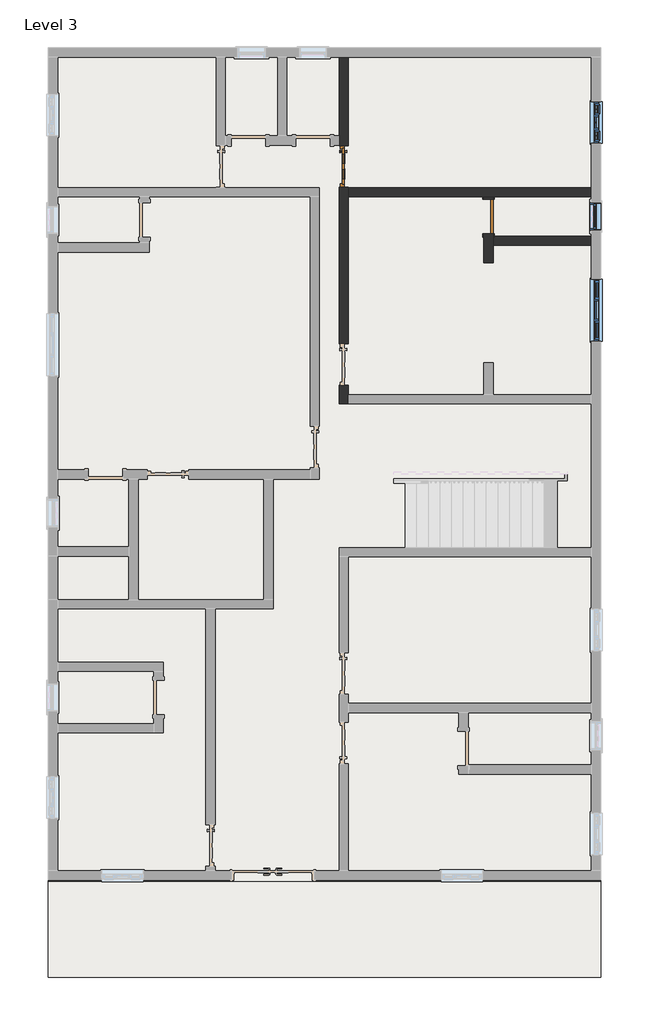
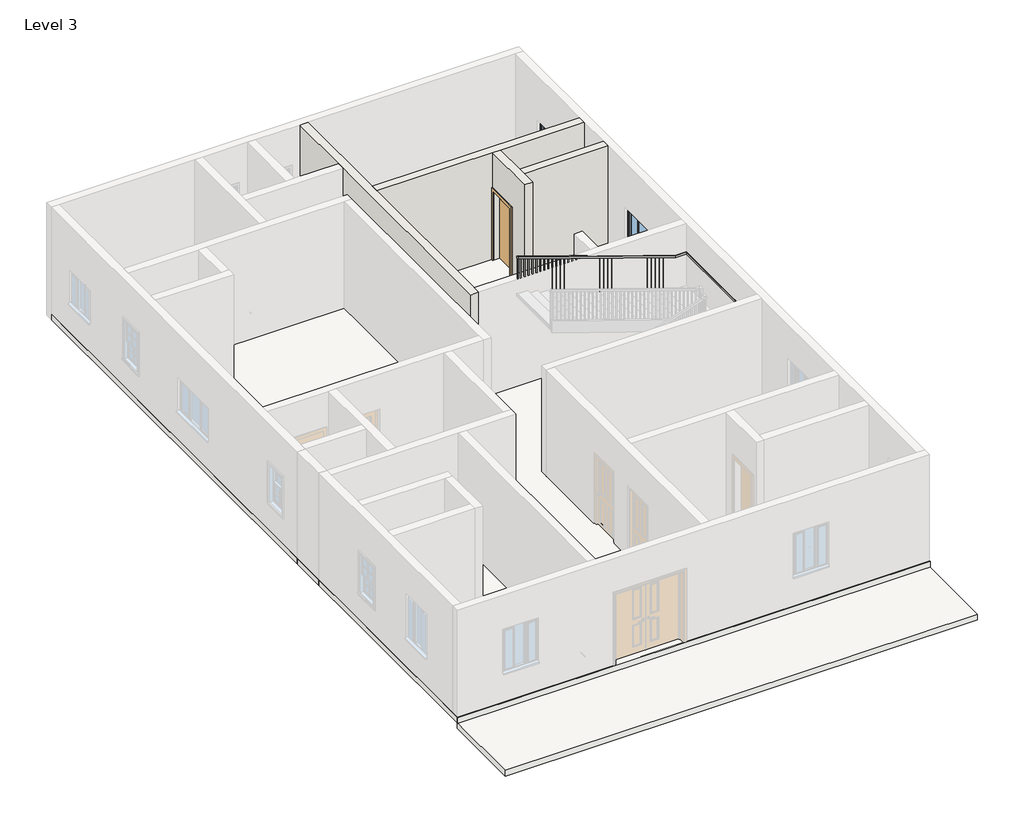
# One storey, part 2 of 3: 4 walls, 3 roofs, 3 windows, 2 doors, 1 railing, 1 slab.
# Revit data of these elements (continued)
# Type "Windows_Tpl_w-Glazing_Cross-Bars : 910x910mm" (continued)
#   Wrap Layers (Int) from Ext = 0' - 6.98819"
#   Window Board Projection = 0' - 0.98425"
#   Window Board Extension = 0' - 0.98425"
#   Visual Light Transmittance = 0.9
#   Solar Heat Gain Coefficient = 0.78
#   Rough Width = 2' - 11.82677"
#   Rough Height = 2' - 11.82677"
#   Height = 2' - 11.82677"
#   Width = 2' - 11.82677"
#   Heat Transfer Coefficient (U) = 0.6496 BTU/(h·ft²·°F)
#   Glazing Thickness = 0' - 0.94488"
#   Glazing Bar Thickness = 0' - 0.7874"
#   FrameOffset - External = 0' - 1.9685"
#   Frame Depth = 0' - 2.55906"
#   Default Head Height = 6' - 11.07087"
#   Cill Depth = 0' - 3.44488"
#   Cavity Closer Width = 0' - 1.9685"
#   Cavity Closer Offset from Ext = 0' - 4.03543"
#   Cavity Closer Depth = 0' - 3.34646"
#   Vis - Glazing Bars = yes
#   Vis - Cavity Closers = yes
#   Define Thermal Properties by = 1
#   Material Trim = Window Frame
#   Material Glazing Bars = Window Frame
#   Material Glass = Glass
#   Material Frame = Window Frame
#   Wall Closure = (empty or 0)
# Element 1 (IfcDoor, "Doors_ExtSgl_2 : 2'x7\"")
#   Phase Created = New Construction
#   Materials on its faces: "Door - Panel", "Door - Handle", "Door - Frame/Mullion", "Door - Glazing"
# Element 2 (IfcDoor, "Single-Flush : 30\" x 80\"")
#   Phase Created = New Construction
#   Materials on its faces: "Door - Frame", "Door - Panel"
# Element 3 (IfcRailing, "Handrail - Rectangular")
#   Phase Created = New Construction
# Elements 4, 5, 6 (IfcRoof, "Generic - 12\"")
#   built-in parameter 1001705 = 20.5 (stored number, unit not read)
#   built-in parameter 1001710 = 33615
#   Phase Created = New Construction
#   Materials on its faces: "Default Roof"
# Element 7 (IfcSlab, "Generic - 12\"")
#   Height Offset From Level = 0' - 0"
#   Phase Created = New Construction
#   Materials on its faces: "Default Floor"
# Elements 8, 9, 10, 11 (IfcWall, "Generic - 4.5\" p")
#   Top Offset = 0' - 0"
#   Base Offset = 0' - 0"
#   Unconnected Height = 10' - 0"
#   wall height = 10' - 0"
#   Phase Created = New Construction
#   Base Constraint = Level 3
#   Materials on its faces: "Default Wall"
# Element 12 (IfcWindow, "Window-Double-Hung : 24\" x 42\"")
#   Mark = "29"
#   Window Inset = 0' - 0"
#   Interior Wall Closure = 0' - 1 1/2"
#   Frame Extension = 0' - 1 1/4"
#   Exterior Wall Closure = 0' - 0 1/2"
#   Interior Trim Visibility = yes
#   Indicator Visibility = yes
#   Exterior Trim Visibility = yes
#   Phase Created = New Construction
#   Materials on its faces: "Wood - Stained", "Glass", "Clad - White"
# Element 13 (IfcWindow, "Windows_Tpl_Plain : 1360x910mm")
#   Mark = "22"
#   Phase Created = New Construction
#   Materials on its faces: "Window Frame", "Glass"
# Element 14 (IfcWindow, "Windows_Tpl_w-Glazing_Cross-Bars : 910x910mm")
#   Mark = "25"
#   Phase Created = New Construction
#   Materials on its faces: "Window Frame", "Glass"
# Materials
#   "Door - Glazing": colour RGB 0 0 255, transparency 0.75
#   "Door - Panel": class "Wood", colour RGB 210 159 95, transparency 0, Cost = 0
#   "Door - Frame/Mullion": class "Wood", colour RGB 212 179 113, transparency 0
#   "Door - Handle": colour RGB 246 240 166, transparency 0
#   "Door - Frame": colour RGB 118 70 51, transparency 0, Cost = 0
#   "Wood - Stained": class "Wood", colour RGB 224 178 126, transparency 0, Cost = 0
#   "Clad - White": class "Wood", colour RGB 242 242 238, transparency 0, Cost = 0
#   "Glass": class "Glass", colour RGB 0 128 192, transparency 0.75, Description = "Soda Lime Glass", Cost = 0
#   "Window Frame": colour RGB 249 249 249, transparency 0
#   "Default Roof": colour RGB 88 101 114, transparency 0, Cost = 0
#   "Default Floor": colour RGB 128 128 128, transparency 0, Cost = 0
#   "Default Wall": colour RGB 128 128 128, transparency 0, Cost = 0
